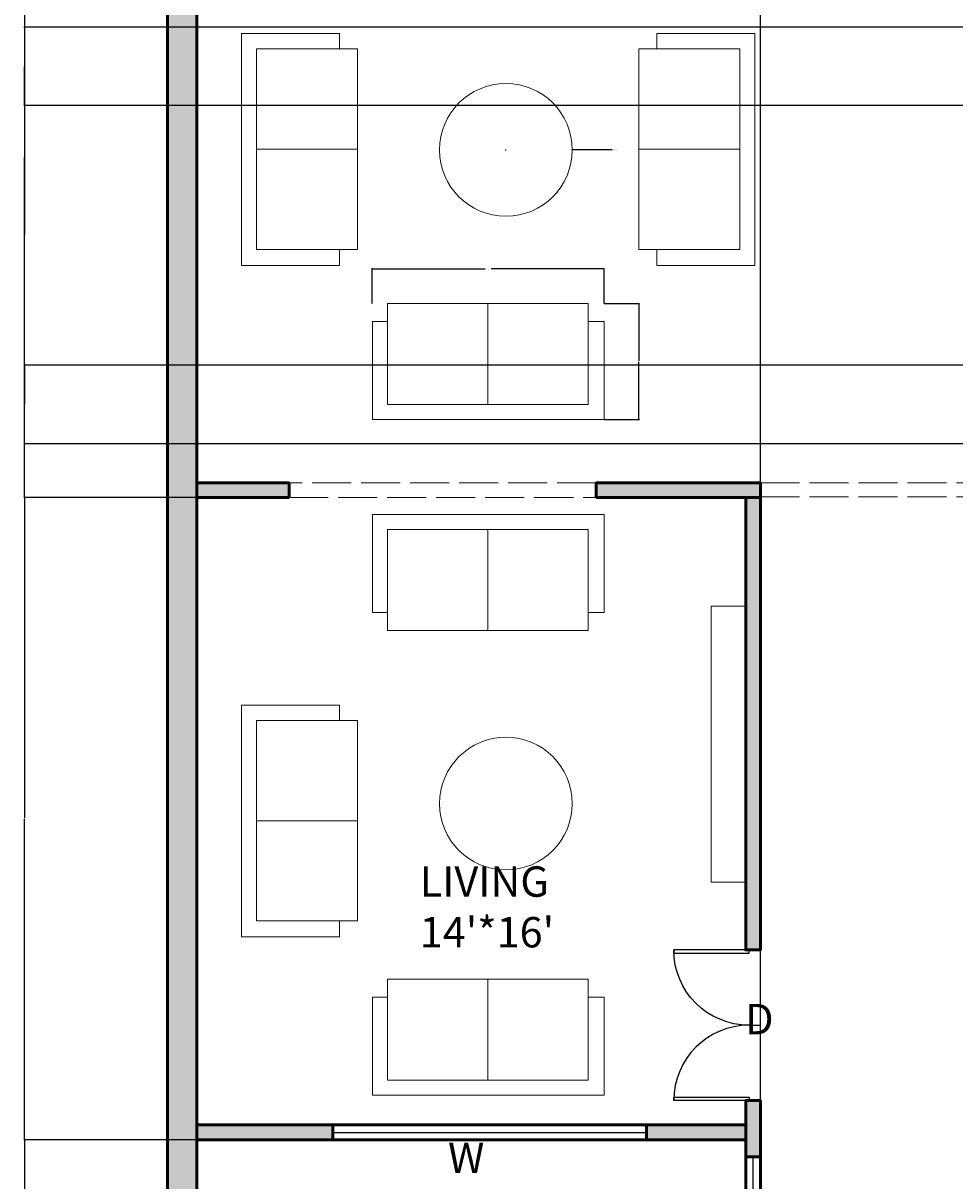
# Model space of a CAD drawing. Units: inches. Extents: x 2024 to 2594, y 643 to 1604.
# Tile 2 of 4: x 2024 to 2309, y 865 to 1219. Entities that reach past the tile are written whole.
import ezdxf

# ---------------------------------------------------------------- set-up
doc = ezdxf.new("R2010")
doc.units = ezdxf.units.IN
doc.linetypes.add('ACAD_ISO02W100', pattern=[15, 12, -3])
for name, color, linetype, lineweight in [('A-ANNO-DIMS', 2, 'Continuous', 18), ('A-ANNO-TEXT', 7, 'Continuous', 18), ('A-AREA-IDEN', 7, 'Continuous', 25), ('A-WALL-OVHD', 50, 'ACAD_ISO02W100', 18), ('A-WALL-PATT', 50, 'Continuous', 13), ('C-PROP', 7, 'Continuous', 35), ('DOOR', 240, 'Continuous', 25), ('FUR', 212, 'Continuous', 18), ('WALL', 50, 'Continuous', 50), ('WIN', 140, 'Continuous', 25)]:
    doc.layers.add(name, color=color, linetype=linetype, lineweight=lineweight)
doc.styles.get("Standard").update_dxf_attribs({"font": 'arial.ttf'})
doc.dimstyles.get("Standard").update_dxf_attribs({"dimtxt": 0.18, "dimasz": 0.18, "dimexe": 0.18, "dimexo": 0.0625, "dimgap": 0.09, "dimtad": 0, "dimtih": 1, "dimtoh": 1, "dimdec": 4, "dimzin": 0, "dimdsep": 46, "dimtxsty": 'Standard', "dimcen": 0.09, "dimadec": 0, "dimazin": 0, "dimtfac": 1, "dimtdec": 4, "dimtofl": 0, "dimtmove": 0, "dimatfit": 3, "dimfxl": 1, "dimtolj": 1, "dimtzin": 0, "dimarcsym": 0})

# ---------------------------------------------------------------- blocks, each defined once
blk = doc.blocks.new('*U2')
for p, q in [((0, 0), (0, -6)), ((40, 0), (40, -6))]:
    blk.add_line(p, q)
blk.add_lwpolyline([(0, 0), (0, 40), (1.75, 40), (1.75, 0)], close=True)
blk.add_arc((0, 0), 40, 0, 90)
blk = doc.blocks.new('SOFA-TWO-SEAT')
for p, q in [((0, 0), (0, 70.94)), ((0, 70.94), (30.01, 70.94)), ((30.01, 70.94), (30.01, 66.25)), ((4.57, 35.56), (35.47, 35.56)), ((30.01, 4.88), (30.01, 0)), ((30.01, 0), (0, 0))]:
    blk.add_line(p, q)
blk.add_lwpolyline([(4.57, 4.88), (35.47, 4.88), (35.47, 66.25), (4.57, 66.25)], close=True)
blk = doc.blocks.new('TABLE-COFFEE-ROUND')
blk.add_circle((20.32, 20.32), 20.32)
blk = doc.blocks.new('*D15')
at = {"layer": 'A-ANNO-DIMS', "color": 0, "lineweight": -2, "transparency": 16777216}
for p, q in [((2130.98, 1133.36), (2130.98, 1144.12)), ((2131.16, 1143.94), (2165.55, 1143.94)), ((2201.75, 1143.94), (2167.36, 1143.94)), ((2201.93, 1133.36), (2201.93, 1144.12))]:
    blk.add_line(p, q, dxfattribs=at)
at = {"layer": 'A-ANNO-DIMS', "color": 0, "lineweight": 100, "transparency": 16777216}
for points in [[(2131.16, 1143.97), (2131.16, 1143.91), (2130.98, 1143.94)], [(2201.75, 1143.97), (2201.75, 1143.91), (2201.93, 1143.94)]]:
    blk.add_solid(points, dxfattribs=at)
at = {"layer": 'Defpoints', "color": 0, "lineweight": 100, "transparency": 16777216}
for p in [(2130.98, 1143.94), (2130.98, 1133.3), (2201.93, 1133.3)]:
    blk.add_point(p, dxfattribs=at)
at = {"layer": 'A-ANNO-DIMS', "color": 0, "transparency": 16777216, "insert": (2166.46, 1143.94), "char_height": 0.18, "attachment_point": 5}
blk.add_mtext('\\A1;SOFA 71 TYP.', dxfattribs=at)
blk = doc.blocks.new('*D16')
at = {"layer": 'A-ANNO-DIMS', "color": 0, "lineweight": -2, "transparency": 16777216}
for p, q in [((2201.99, 1133.3), (2212.75, 1133.3)), ((2212.57, 1133.12), (2212.57, 1115.75)), ((2212.57, 1098.01), (2212.57, 1115.38)), ((2201.99, 1097.83), (2212.75, 1097.83))]:
    blk.add_line(p, q, dxfattribs=at)
at = {"layer": 'A-ANNO-DIMS', "color": 0, "lineweight": 100, "transparency": 16777216}
for points in [[(2212.54, 1133.12), (2212.6, 1133.12), (2212.57, 1133.3)], [(2212.54, 1098.01), (2212.6, 1098.01), (2212.57, 1097.83)]]:
    blk.add_solid(points, dxfattribs=at)
at = {"layer": 'Defpoints', "color": 0, "lineweight": 100, "transparency": 16777216}
for p in [(2201.93, 1133.3), (2212.57, 1133.3), (2201.93, 1097.83)]:
    blk.add_point(p, dxfattribs=at)
at = {"layer": 'A-ANNO-DIMS', "color": 0, "transparency": 16777216, "insert": (2212.57, 1115.56), "char_height": 0.18, "attachment_point": 5}
blk.add_mtext('\\A1;35 TYP.', dxfattribs=at)
blk = doc.blocks.new('*D32')
at = {"layer": 'A-ANNO-DIMS', "color": 0, "lineweight": -2, "transparency": 16777216}
for p, q in [((2077.21, 877.43), (2024.29, 877.43)), ((2024.47, 877.25), (2024.47, 811.73)), ((2024.47, 745.85), (2024.47, 811.37)), ((2245.21, 745.67), (2024.29, 745.67))]:
    blk.add_line(p, q, dxfattribs=at)
at = {"layer": 'A-ANNO-DIMS', "color": 0, "lineweight": 100, "transparency": 16777216}
for points in [[(2024.44, 877.25), (2024.5, 877.25), (2024.47, 877.43)], [(2024.44, 745.85), (2024.5, 745.85), (2024.47, 745.67)]]:
    blk.add_solid(points, dxfattribs=at)
at = {"layer": 'Defpoints', "color": 0, "lineweight": 100, "transparency": 16777216}
for p in [(2024.47, 877.43), (2077.27, 877.43), (2245.27, 745.67)]:
    blk.add_point(p, dxfattribs=at)
at = {"layer": 'A-ANNO-DIMS', "color": 0, "transparency": 16777216, "insert": (2024.47, 811.55), "char_height": 0.18, "attachment_point": 5}
blk.add_mtext('\\A1;131.76', dxfattribs=at)
blk = doc.blocks.new('*D33')
at = {"layer": 'A-ANNO-DIMS', "color": 0, "lineweight": -2, "transparency": 16777216}
for p, q in [((2077.21, 1073.92), (2024.29, 1073.92)), ((2024.47, 1073.74), (2024.47, 975.86)), ((2024.47, 877.61), (2024.47, 975.49)), ((2077.21, 877.43), (2024.29, 877.43))]:
    blk.add_line(p, q, dxfattribs=at)
at = {"layer": 'A-ANNO-DIMS', "color": 0, "lineweight": 100, "transparency": 16777216}
for points in [[(2024.44, 1073.74), (2024.5, 1073.74), (2024.47, 1073.92)], [(2024.44, 877.61), (2024.5, 877.61), (2024.47, 877.43)]]:
    blk.add_solid(points, dxfattribs=at)
at = {"layer": 'Defpoints', "color": 0, "lineweight": 100, "transparency": 16777216}
for p in [(2024.47, 1073.92), (2077.27, 1073.92), (2077.27, 877.43)]:
    blk.add_point(p, dxfattribs=at)
at = {"layer": 'A-ANNO-DIMS', "color": 0, "transparency": 16777216, "insert": (2024.47, 975.68), "char_height": 0.18, "attachment_point": 5}
blk.add_mtext('\\A1;196.5', dxfattribs=at)
blk = doc.blocks.new('*D34')
at = {"layer": 'A-ANNO-DIMS', "color": 0, "lineweight": -2, "transparency": 16777216}
for p, q in [((2077.21, 1282.43), (2024.29, 1282.43)), ((2024.47, 1282.25), (2024.47, 1178.36)), ((2024.47, 1074.1), (2024.47, 1177.99)), ((2077.21, 1073.92), (2024.29, 1073.92))]:
    blk.add_line(p, q, dxfattribs=at)
at = {"layer": 'A-ANNO-DIMS', "color": 0, "lineweight": 100, "transparency": 16777216}
for points in [[(2024.44, 1282.25), (2024.5, 1282.25), (2024.47, 1282.43)], [(2024.44, 1074.1), (2024.5, 1074.1), (2024.47, 1073.92)]]:
    blk.add_solid(points, dxfattribs=at)
at = {"layer": 'Defpoints', "color": 0, "lineweight": 100, "transparency": 16777216}
for p in [(2024.47, 1282.43), (2077.27, 1282.43), (2077.27, 1073.92)]:
    blk.add_point(p, dxfattribs=at)
at = {"layer": 'A-ANNO-DIMS', "color": 0, "transparency": 16777216, "insert": (2024.47, 1178.18), "char_height": 0.18, "attachment_point": 5}
blk.add_mtext('\\A1;208.5', dxfattribs=at)
blk = doc.blocks.new('*D42')
at = {"layer": 'A-ANNO-DIMS', "color": 0, "lineweight": -2, "transparency": 16777216}
for p, q in [((2326.21, 1114.43), (2024.29, 1114.43)), ((2024.47, 1114.25), (2024.47, 1102.61)), ((2024.47, 1090.61), (2024.47, 1102.25)), ((2326.21, 1090.43), (2024.29, 1090.43))]:
    blk.add_line(p, q, dxfattribs=at)
at = {"layer": 'A-ANNO-DIMS', "color": 0, "lineweight": 100, "transparency": 16777216}
for points in [[(2024.44, 1114.25), (2024.5, 1114.25), (2024.47, 1114.43)], [(2024.44, 1090.61), (2024.5, 1090.61), (2024.47, 1090.43)]]:
    blk.add_solid(points, dxfattribs=at)
at = {"layer": 'Defpoints', "color": 0, "lineweight": 100, "transparency": 16777216}
for p in [(2024.47, 1114.43), (2326.27, 1114.43), (2326.27, 1090.43)]:
    blk.add_point(p, dxfattribs=at)
at = {"layer": 'A-ANNO-DIMS', "color": 0, "transparency": 16777216, "insert": (2024.47, 1102.43), "char_height": 0.18, "attachment_point": 5}
blk.add_mtext('\\A1;24', dxfattribs=at)
blk = doc.blocks.new('*D43')
at = {"layer": 'A-ANNO-DIMS', "color": 0, "lineweight": -2, "transparency": 16777216}
for p, q in [((2326.21, 1193.93), (2024.29, 1193.93)), ((2024.47, 1193.75), (2024.47, 1154.36)), ((2024.47, 1114.61), (2024.47, 1154)), ((2326.21, 1114.43), (2024.29, 1114.43))]:
    blk.add_line(p, q, dxfattribs=at)
at = {"layer": 'A-ANNO-DIMS', "color": 0, "lineweight": 100, "transparency": 16777216}
for points in [[(2024.44, 1193.75), (2024.5, 1193.75), (2024.47, 1193.93)], [(2024.44, 1114.61), (2024.5, 1114.61), (2024.47, 1114.43)]]:
    blk.add_solid(points, dxfattribs=at)
at = {"layer": 'Defpoints', "color": 0, "lineweight": 100, "transparency": 16777216}
for p in [(2024.47, 1193.93), (2326.27, 1193.93), (2326.27, 1114.43)]:
    blk.add_point(p, dxfattribs=at)
at = {"layer": 'A-ANNO-DIMS', "color": 0, "transparency": 16777216, "insert": (2024.47, 1154.18), "char_height": 0.18, "attachment_point": 5}
blk.add_mtext('\\A1;79.5', dxfattribs=at)
blk = doc.blocks.new('*D44')
at = {"layer": 'A-ANNO-DIMS', "color": 0, "lineweight": -2, "transparency": 16777216}
for p, q in [((2326.21, 1217.93), (2024.29, 1217.93)), ((2024.47, 1217.75), (2024.47, 1206.11)), ((2024.47, 1194.11), (2024.47, 1205.75)), ((2326.21, 1193.93), (2024.29, 1193.93))]:
    blk.add_line(p, q, dxfattribs=at)
at = {"layer": 'A-ANNO-DIMS', "color": 0, "lineweight": 100, "transparency": 16777216}
for points in [[(2024.44, 1217.75), (2024.5, 1217.75), (2024.47, 1217.93)], [(2024.44, 1194.11), (2024.5, 1194.11), (2024.47, 1193.93)]]:
    blk.add_solid(points, dxfattribs=at)
at = {"layer": 'Defpoints', "color": 0, "lineweight": 100, "transparency": 16777216}
for p in [(2024.47, 1217.93), (2326.27, 1217.93), (2326.27, 1193.93)]:
    blk.add_point(p, dxfattribs=at)
at = {"layer": 'A-ANNO-DIMS', "color": 0, "transparency": 16777216, "insert": (2024.47, 1205.93), "char_height": 0.18, "attachment_point": 5}
blk.add_mtext('\\A1;24', dxfattribs=at)
blk = doc.blocks.new('*D48')
at = {"layer": 'A-ANNO-DIMS', "color": 0, "lineweight": -2, "transparency": 16777216}
for p, q in [((2249.77, 819.02), (2249.77, 1603.82)), ((2249.95, 1603.64), (2299.2, 1603.64)), ((2349.09, 1603.64), (2299.85, 1603.64)), ((2349.27, 860.99), (2349.27, 1603.82))]:
    blk.add_line(p, q, dxfattribs=at)
at = {"layer": 'A-ANNO-DIMS', "color": 0, "lineweight": 100, "transparency": 16777216}
for points in [[(2249.95, 1603.67), (2249.95, 1603.61), (2249.77, 1603.64)], [(2349.09, 1603.67), (2349.09, 1603.61), (2349.27, 1603.64)]]:
    blk.add_solid(points, dxfattribs=at)
at = {"layer": 'Defpoints', "color": 0, "lineweight": 100, "transparency": 16777216}
for p in [(2349.27, 1603.64), (2349.27, 860.93), (2249.77, 818.96)]:
    blk.add_point(p, dxfattribs=at)
at = {"layer": 'A-ANNO-DIMS', "color": 0, "transparency": 16777216, "insert": (2299.52, 1603.64), "char_height": 0.18, "attachment_point": 5}
blk.add_mtext('\\A1;99.5', dxfattribs=at)
blk = doc.blocks.new('*D57')
at = {"layer": 'A-ANNO-DIMS', "color": 0, "lineweight": -2, "transparency": 16777216}
for p, q in [((2171.78, 1180.35), (2171.96, 1180.35)), ((2171.87, 1180.26), (2171.87, 1180.44)), ((2204.38, 1180.35), (2192.37, 1180.35))]:
    blk.add_line(p, q, dxfattribs=at)
at = {"layer": 'A-ANNO-DIMS', "color": 0, "lineweight": 100, "transparency": 16777216}
blk.add_solid([(2192.37, 1180.38), (2192.37, 1180.32), (2192.19, 1180.35)], dxfattribs=at)
at = {"layer": 'Defpoints', "color": 0, "lineweight": 100, "transparency": 16777216}
for p in [(2151.56, 1180.35), (2192.19, 1180.35)]:
    blk.add_point(p, dxfattribs=at)
at = {"layer": 'A-ANNO-DIMS', "color": 0, "transparency": 16777216, "insert": (2205.07, 1180.35), "char_height": 0.18, "attachment_point": 5}
blk.add_mtext('\\A1;2X ∅40.64', dxfattribs=at)

msp = doc.modelspace()

# ---------------------------------------------------------------- hatches: boundary and pattern name
at = {"layer": 'A-WALL-PATT'}
h = msp.add_hatch(color=256, dxfattribs=at)
h.dxf.hatch_style = 1
h.paths.add_polyline_path([(2543.7727, 1526.9303), (2077.2727, 1526.9303), (2077.2727, 1522.4303), (2543.7727, 1522.4303)])
h.paths.add_polyline_path([(2077.2727, 1526.9303), (2068.2727, 1526.9303), (2068.2727, 1475.9303), (2077.2727, 1475.9303)])
h.paths.add_polyline_path([(2077.2727, 1475.9303), (2068.2727, 1475.9303), (2068.2727, 686.9303), (2077.2727, 686.9303)])
h.paths.add_polyline_path([(2548.2727, 1526.9303), (2543.7727, 1526.9303), (2543.7727, 1522.4303), (2543.7727, 691.4303), (2548.2727, 691.4303)])
h.paths.add_polyline_path([(2249.7727, 1078.4303), (2199.5227, 1078.4303), (2199.5227, 1073.9303), (2245.2727, 1073.9303), (2249.7727, 1073.9217)])
h.paths.add_polyline_path([(2249.7727, 1073.9217), (2245.2727, 1073.9217), (2245.2727, 935.5102), (2249.7727, 935.5102)])
h.paths.add_polyline_path([(2326.2727, 1121.201), (2321.7727, 1121.201), (2321.7727, 1085.9303), (2326.2727, 1085.9303), (2326.2727, 1090.4303)])
h.paths.add_polyline_path([(2497.2727, 1090.4303), (2326.2727, 1090.4303), (2326.2727, 1085.9303), (2497.2727, 1085.9303)])
h.paths.add_polyline_path([(2326.2727, 1085.9303), (2321.7727, 1085.9303), (2321.7727, 989.0099), (2326.2727, 989.0099)])
h.paths.add_polyline_path([(2199.1605, 1286.9303), (2077.2727, 1286.9303), (2077.2727, 1282.4303), (2199.1605, 1282.4303)])
h.paths.add_polyline_path([(2321.7727, 1286.9303), (2239.1605, 1286.9303), (2239.1605, 1282.4303), (2321.7727, 1282.4303)])
h.paths.add_polyline_path([(2245.2727, 881.9303), (2214.9534, 881.9303), (2214.9534, 877.4303), (2245.2727, 877.4303)])
h.paths.add_polyline_path([(2118.9166, 881.9303), (2077.2727, 881.9303), (2077.2727, 877.4303), (2118.9166, 877.4303)])
h.paths.add_polyline_path([(2249.7727, 889.4074), (2246.315, 889.4074), (2245.2727, 889.4074), (2245.2727, 872.2078), (2249.7727, 872.2078)])
h.paths.add_polyline_path([(2405.0472, 941.9303), (2326.2727, 941.9303), (2326.2727, 937.4303), (2405.0472, 937.4303)])
h.paths.add_polyline_path([(2326.2727, 949.0099), (2321.7727, 949.0099), (2321.7727, 902.6727), (2326.2727, 902.6727)])
h.paths.add_polyline_path([(2326.2727, 871.366), (2321.7727, 871.366), (2321.7727, 865.4303), (2326.2727, 865.4303)])
h.paths.add_polyline_path([(2401.2727, 937.4303), (2396.7727, 937.4303), (2396.7727, 865.4303), (2401.2727, 865.4303)])
h.paths.add_polyline_path([(2497.2727, 941.9303), (2436.2168, 941.9303), (2436.2168, 937.4303), (2497.2727, 937.4303)])
h.paths.add_polyline_path([(2506.2727, 977.6959), (2497.2727, 977.6959), (2497.2727, 745.6665), (2506.2727, 745.6665)])
h.paths.add_polyline_path([(2497.2727, 754.6665), (2309.6667, 754.6665), (2309.6667, 745.6665), (2497.2727, 745.6665)])
h.paths.add_polyline_path([(2258.2092, 754.6665), (2245.2727, 754.6665), (2245.2727, 745.6665), (2258.2092, 745.6665)])
h.paths.add_polyline_path([(2249.7727, 772.853), (2248.7304, 772.853), (2245.2727, 772.853), (2245.2727, 754.6665), (2249.7727, 754.6665)])
h.paths.add_polyline_path([(2249.7727, 825.5234), (2245.2727, 825.5234), (2245.2727, 818.9558), (2248.7304, 818.9558), (2249.7727, 818.9558)])
h.paths.add_polyline_path([(2105.513, 1078.4303), (2077.2727, 1078.4303), (2077.2727, 1073.9303), (2105.513, 1073.9303)])
h.paths.add_polyline_path([(2326.2727, 1466.9303), (2321.7727, 1466.9303), (2321.7727, 1267.3126), (2326.2727, 1267.3126)])
h.paths.add_polyline_path([(2405.7727, 1466.9303), (2401.2727, 1466.9303), (2401.2727, 1438.953), (2405.7727, 1438.953)])
h.paths.add_polyline_path([(2405.7727, 1398.953), (2401.2727, 1398.953), (2401.2727, 1394.9303), (2405.7727, 1394.9303)])
h.paths.add_polyline_path([(2467.5339, 860.9303), (2467.5339, 865.4303), (2321.7727, 865.4303), (2321.7727, 860.9303)])
h.paths.add_polyline_path([(2488.7331, 865.4303), (2488.7331, 860.9303), (2497.2727, 860.9303), (2497.2727, 865.4303)])

# ---------------------------------------------------------------- linework, layer by layer
at = {"layer": 'A-WALL-OVHD'}
for points in [[(2105.513, 1073.9217), (2199.5227, 1073.9217), (2199.5227, 1078.4303), (2105.513, 1078.4303)], [(2249.7727, 1078.4303), (2321.7727, 1078.4303), (2321.7727, 1074.2238), (2249.7727, 1074.2238)]]:
    msp.add_lwpolyline(points, close=True, dxfattribs=at)
at = {"layer": 'C-PROP'}
msp.add_line((2068.2727, 686.9303), (2068.2727, 1526.9303), dxfattribs=at)
msp.add_lwpolyline([(2548.2727, 686.9303), (2068.2727, 686.9303), (2068.2727, 1526.9303), (2548.2727, 1526.9303)], close=True, dxfattribs=at)
at = {"layer": 'FUR'}
msp.add_lwpolyline([(2245.2727, 956.2611), (2234.7548, 956.2611), (2234.7548, 1040.7121), (2245.2727, 1040.7121)], close=True, dxfattribs=at)
at = {"layer": 'WALL'}
for p, q in [((2077.2727, 1282.4303), (2077.2727, 1078.4303)), ((2077.2727, 1078.4303), (2105.513, 1078.4303)), ((2105.513, 1073.9303), (2105.513, 1078.4303)), ((2199.5227, 1073.9303), (2199.5227, 1078.4303)), ((2199.5227, 1078.4303), (2249.7727, 1078.4303)), ((2249.7727, 1073.9303), (2249.7727, 1078.4303)), ((2077.2727, 1073.9303), (2105.513, 1073.9303)), ((2077.2727, 1073.9303), (2077.2727, 881.9303)), ((2199.5227, 1073.9303), (2245.2727, 1073.9303)), ((2245.2727, 935.5102), (2245.2727, 1073.9303)), ((2249.7727, 935.5102), (2249.7727, 1073.9303)), ((2245.2727, 912.4353), (2245.2727, 912.4824)), ((2245.2727, 881.9303), (2245.2727, 889.4074)), ((2249.7727, 877.4303), (2249.7727, 889.4074)), ((2077.2727, 881.9303), (2245.2727, 881.9303)), ((2077.2727, 877.4303), (2245.2727, 877.4303)), ((2245.2727, 877.4303), (2245.2727, 818.9558)), ((2249.7727, 877.4303), (2249.7727, 818.9558))]:
    msp.add_line(p, q, dxfattribs=at)
for points in [[(2077.2727, 881.9303), (2077.2727, 1517.9303)], [(2077.2727, 695.9303), (2077.2727, 877.4303)]]:
    msp.add_lwpolyline(points, dxfattribs=at)
for points in [[(2068.2727, 1475.9303), (2077.2727, 1475.9303), (2077.2727, 686.9303), (2068.2727, 686.9303)], [(2105.513, 1073.9217), (2077.2727, 1073.9217), (2077.2727, 1078.4303), (2105.513, 1078.4303)], [(2199.5227, 1073.9217), (2249.7727, 1073.9217), (2249.7727, 1078.4303), (2199.5227, 1078.4303)], [(2249.7727, 1073.9217), (2245.2727, 1073.9217), (2245.2727, 935.5102), (2249.7727, 935.5102)], [(2245.2727, 872.2078), (2249.7727, 872.2078), (2249.7727, 889.4074), (2245.2727, 889.4074)], [(2118.9166, 881.9303), (2077.2727, 881.9303), (2077.2727, 877.4303), (2118.9166, 877.4303)], [(2214.9534, 877.4303), (2245.2727, 877.4303), (2245.2727, 881.9303), (2214.9534, 881.9303)]]:
    msp.add_lwpolyline(points, close=True, dxfattribs=at)
at = {"layer": 'WIN'}
for p, q in [((2118.9166, 879.6803), (2214.9534, 879.6803)), ((2247.5227, 825.5234), (2247.5227, 872.2078))]:
    msp.add_line(p, q, dxfattribs=at)
for points in [[(2118.9166, 877.4303), (2214.9534, 877.4303), (2214.9534, 881.9303), (2118.9166, 881.9303)], [(2245.2727, 825.5234), (2249.7727, 825.5234), (2249.7727, 872.2078), (2245.2727, 872.2078)]]:
    msp.add_lwpolyline(points, close=True, dxfattribs=at)

# ---------------------------------------------------------------- block references
at = {"layer": 'DOOR', "yscale": 0.5762850341581635, "zscale": 0.5762850341581635}
for p, xscale, rotation in [((2246.315, 935.5102), -0.5762850341581635, 90), ((2246.315, 889.4074), 0.5762850341581635, 90.00000000000003)]:
    msp.add_blockref('*U2', p, dxfattribs=dict(at, xscale=xscale, rotation=rotation))
at = {"layer": 'FUR'}
for name, p in [('SOFA-TWO-SEAT', (2090.956, 1144.9872)), ('TABLE-COFFEE-ROUND', (2151.557, 1160.0336)), ('SOFA-TWO-SEAT', (2090.956, 939.486)), ('TABLE-COFFEE-ROUND', (2151.557, 959.978))]:
    msp.add_blockref(name, p, dxfattribs=at)
at = {"layer": 'FUR', "extrusion": (0, 0, -1), "zscale": -1}
msp.add_blockref('SOFA-TWO-SEAT', (-2248.0692, 1144.9872), dxfattribs=at)
at = {"layer": 'FUR'}
for p, rotation in [((2201.9276, 1097.8311), 90.00000000000146), ((2201.9276, 891.0576), 89.99999999999991)]:
    msp.add_blockref('SOFA-TWO-SEAT', p, dxfattribs=dict(at, rotation=rotation))
at = {"layer": 'FUR', "extrusion": (0, 0, -1), "zscale": -1, "rotation": 270.0000000000003}
msp.add_blockref('SOFA-TWO-SEAT', (-2201.9276, 1068.765), dxfattribs=at)

# ---------------------------------------------------------------- texts
at = {"layer": 'A-ANNO-TEXT', "char_height": 9.3008, "attachment_point": 1}
for s, insert in [('D', (2245.096, 918.9763)), ('W', (2154.1413, 876.5481))]:
    msp.add_mtext_dynamic_manual_height_columns(s, width=384.915388, gutter_width=46.5039, heights=[0], dxfattribs=dict(at, insert=insert))
at = {"layer": 'A-AREA-IDEN', "insert": (2145.4975, 961.0845), "char_height": 9.30079, "attachment_point": 1}
msp.add_mtext_dynamic_manual_height_columns("LIVING\\P14'*16'", width=384.915388, gutter_width=46.5039, heights=[0], dxfattribs=at)

# ---------------------------------------------------------------- dimensions: what is measured, and where the dimension line sits
at = {"layer": 'A-ANNO-DIMS'}
dim = msp.add_linear_dim(base=(2349.2727, 1603.6424), p1=(2249.7727, 818.9558), p2=(2349.2727, 860.9303), dimstyle='Standard', override={"dimdec": 1, "dimlfac": 1, "dimrnd": 0, "dimzin": 0, "dimdsep": 46, "dimlunit": 2}, dxfattribs=at)
dim.commit()
dim.dimension.update_dxf_attribs({"geometry": '*D48', "text_midpoint": (2299.5227, 1603.6424)})
for base, p1, p2, override, picture, middle in [((2024.4727, 1282.4303), (2077.2727, 1073.9217), (2077.2727, 1282.4303), {"dimdec": 1, "dimlfac": 1, "dimrnd": 0, "dimzin": 0, "dimdsep": 46, "dimlunit": 2}, '*D34', (2024.4727, 1178.176)), ((2024.4727, 1217.9303), (2326.2727, 1193.9303), (2326.2727, 1217.9303), {"dimdec": 0, "dimlfac": 1, "dimrnd": 0, "dimzin": 0, "dimdsep": 46, "dimlunit": 2}, '*D44', (2024.4727, 1205.9303)), ((2024.4727, 1193.9303), (2326.2727, 1114.4303), (2326.2727, 1193.9303), {"dimdec": 1, "dimlfac": 1, "dimrnd": 0, "dimzin": 0, "dimdsep": 46, "dimlunit": 2}, '*D43', (2024.4727, 1154.1803)), ((2024.4727, 1114.4303), (2326.2727, 1090.4303), (2326.2727, 1114.4303), {"dimdec": 0, "dimlfac": 1, "dimrnd": 0, "dimzin": 0, "dimdsep": 46, "dimlunit": 2}, '*D42', (2024.4727, 1102.4303)), ((2024.4727, 1073.9217), (2077.2727, 877.4303), (2077.2727, 1073.9217), {"dimdec": 1, "dimlfac": 1, "dimrnd": 0, "dimzin": 0, "dimdsep": 46, "dimlunit": 2}, '*D33', (2024.4727, 975.676)), ((2024.4727, 877.4303), (2245.2727, 745.6665), (2077.2727, 877.4303), {"dimdec": 2, "dimlfac": 1, "dimrnd": 0, "dimzin": 0, "dimdsep": 46, "dimlunit": 2}, '*D32', (2024.4727, 811.5484))]:
    dim = msp.add_linear_dim(base=base, p1=p1, p2=p2, angle=90, dimstyle='Standard', override=override, dxfattribs=at)
    dim.commit()
    dim.dimension.update_dxf_attribs({"geometry": picture, "text_midpoint": middle})
dim = msp.add_diameter_dim_2p(p1=(2151.5568, 1180.3521), p2=(2192.193, 1180.352), text='2X <>', dimstyle='Standard', override={"dimdec": 2, "dimlfac": 1, "dimrnd": 0, "dimzin": 0, "dimdsep": 46, "dimlunit": 2}, dxfattribs=at)
dim.commit()
dim.dimension.update_dxf_attribs({"geometry": '*D57', "text_midpoint": (2204.3838, 1180.352), "dimtype": 163})
for base, p1, p2, angle, text, picture, middle in [((2130.9842, 1143.94), (2201.9281, 1133.2984), (2130.9842, 1133.2984), 180, 'SOFA <> TYP.', '*D15', (2166.4561, 1143.94)), ((2212.5696, 1133.2984), (2201.9281, 1097.831), (2201.9281, 1133.2984), 90, '<> TYP.', '*D16', (2212.5696, 1115.5647))]:
    dim = msp.add_linear_dim(base=base, p1=p1, p2=p2, angle=angle, text=text, dimstyle='Standard', override={"dimdec": 0, "dimlfac": 1, "dimrnd": 0, "dimzin": 0, "dimdsep": 46, "dimlunit": 2}, dxfattribs=at)
    dim.commit()
    dim.dimension.update_dxf_attribs({"geometry": picture, "text_midpoint": middle})

doc.saveas('drawing.dxf')
